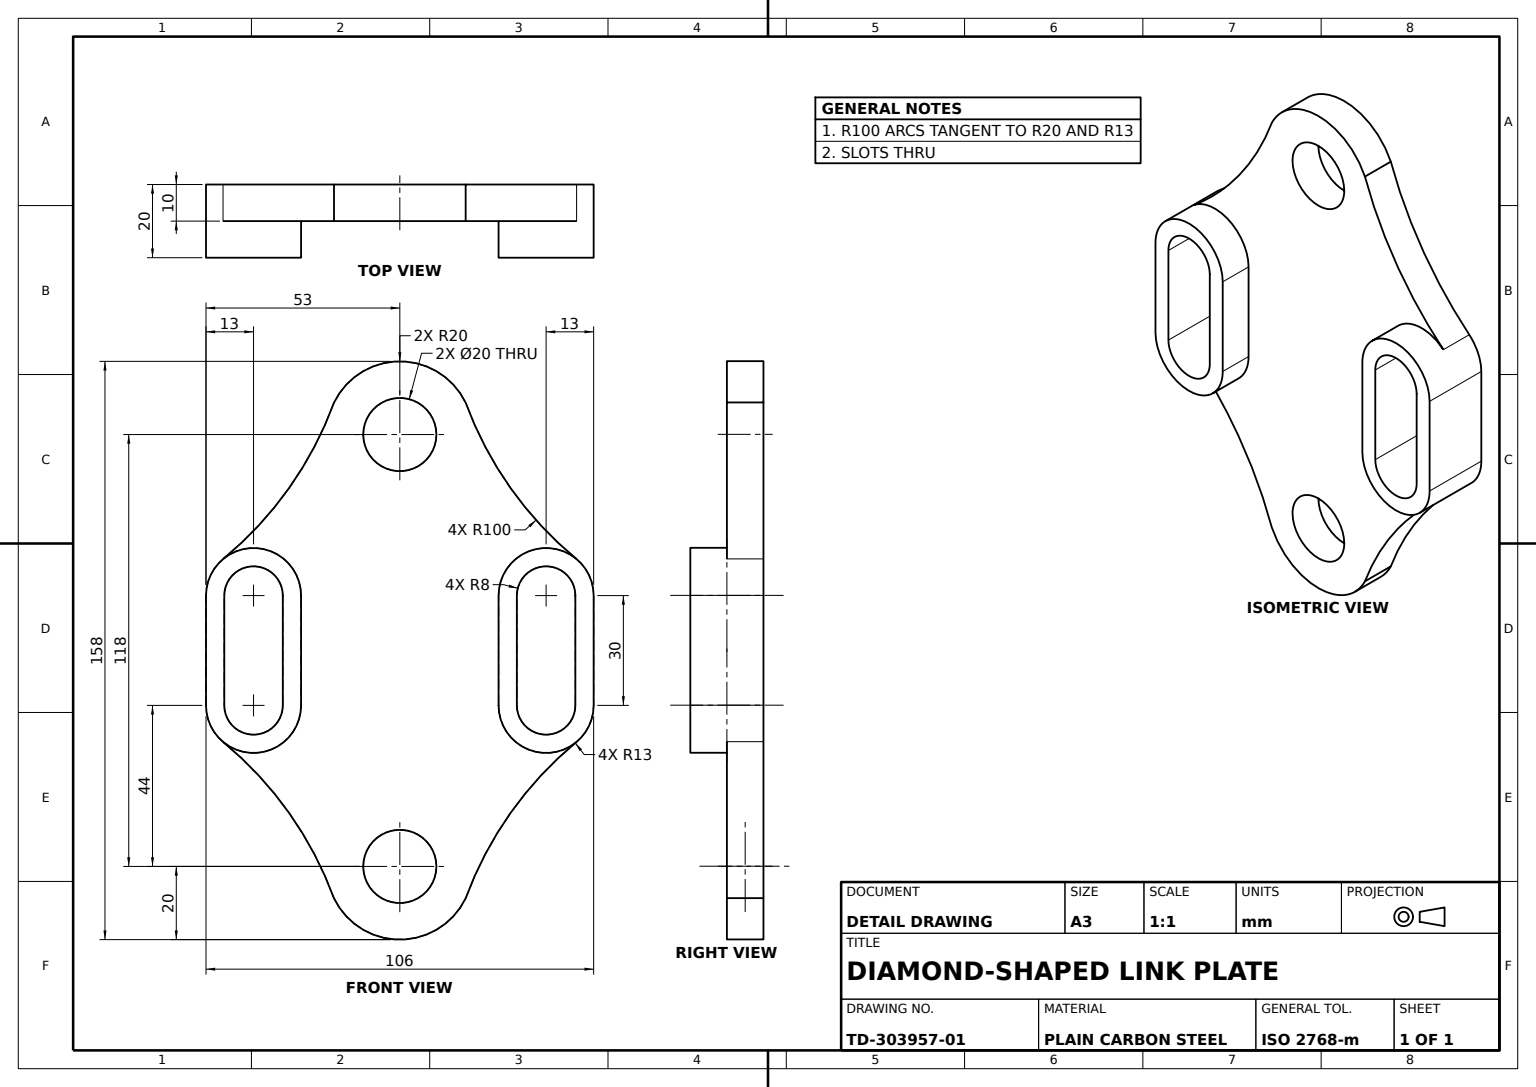
SolidWorks part; units mm, degrees
material "Plain Carbon Steel"
ref_plane "Front Plane" through (0, 0, 0) normal (0, 0, 1) x (1, 0, 0)
ref_plane "Top Plane" through (0, 0, 0) normal (0, 1, 0) x (1, 0, 0)
ref_plane "Right Plane" through (0, 0, 0) normal (1, 0, 0) x (0, 0, -1)
sketch "Diamond Plate Profile" plane through (0, 0, 0) normal (0, 0, 1) x (1, 0, 0)
  line L6 (53, -74) -> (53, -44)
  line L8 (-53, -44) -> (-53, -74)
  arc A0 (17.9996, 8.7185) -> (-17.9996, 8.7185) centre (0, 0) ccw
  arc A1 (-17.9996, -126.7185) -> (17.9996, -126.7185) centre (0, -118) ccw
  arc A2 (53, -44) -> (48.341, -34.0287) centre (40, -44) ccw
  arc A3 (48.341, -83.9713) -> (53, -74) centre (40, -74) ccw
  arc A4 (-48.341, -34.0287) -> (-53, -44) centre (-40, -44) ccw
  arc A5 (-53, -74) -> (-48.1941, -84.0924) centre (-40, -74) ccw
  arc A6 (17.9996, 8.7185) -> (48.341, -34.0287) centre (111.866, 43.202) ccw
  arc A7 (-17.9996, 8.7185) -> (-48.341, -34.0287) centre (-111.866, 43.202) cw
  arc A8 (-17.9996, -126.7185) -> (-48.341, -83.9713) centre (-111.866, -161.202) ccw
  arc A9 (17.9996, -126.7185) -> (48.341, -83.9713) centre (111.866, -161.202) cw
  dimension "D1" = 20
  dimension "D2" = 13
  dimension "D3" = 100
  dimension "D4" = 4.659
  dimension "D5" = 35.0004
  dimension "D6" = 53
  dimension "D7" = 164.866
  dimension "D8" = 117.202
extrude "Diamond Plate" add sketch "Diamond Plate Profile" along normal blind 10 contours A1 A9 A3 L6 A2 A6 A0 A7 A4 L8 A5 A8
sketch "Slot Cuts Profile" plane through (0, 0, 10) normal (0, 0, 1) x (1, 0, 0)
  line L0 (-48, -44) -> (-48, -74)
  line L1 (32, -44) -> (32, -74)
  line L2 (-32, -74) -> (-32, -44)
  line L4 (48, -74) -> (48, -44)
  arc A0 (-32, -44) -> (-48, -44) centre (-40, -44) ccw
  arc A2 (48, -44) -> (32, -44) centre (40, -44) ccw
  arc A3 (32, -74) -> (48, -74) centre (40, -74) ccw
  arc A4 (-48, -74) -> (-32, -74) centre (-40, -74) ccw
  dimension "D1" = 8
extrude "Through Slots 2x" cut sketch "Slot Cuts Profile" against normal blind 10
sketch "Slot Boss A Profile" plane through (0, 0, 10) normal (0, 0, 1) x (1, 0, 0)
  line L0 (-27, -44) -> (-27, -74)
  line L2 (-53, -74) -> (-53, -44)
  line L3 (-32, -44) -> (-32, -74)
  line L4 (-48, -44) -> (-48, -74)
  arc A0 (-27, -44) -> (-53, -44) centre (-40, -44) ccw
  arc A1 (-53, -74) -> (-27, -74) centre (-40, -74) ccw
  arc A2 (-32, -44) -> (-48, -44) centre (-40, -44) ccw
  arc A3 (-48, -74) -> (-32, -74) centre (-40, -74) ccw
extrude "Slot Boss A" add sketch "Slot Boss A Profile" along normal blind 10
sketch "End Holes Profile" plane through (0, 0, 10) normal (0, 0, 1) x (1, 0, 0)
  circle A0 centre (0, 0) radius 10
  circle A1 centre (0, -118) radius 10
  dimension "D1" = 20
extrude "End Holes 2x" cut sketch "End Holes Profile" against normal blind 10
sketch "Slot Boss B Profile" plane through (0, 0, 10) normal (0, 0, 1) x (1, 0, 0)
  line L0 (27, -44) -> (27, -74)
  line L2 (53, -74) -> (53, -44)
  line L3 (32, -44) -> (32, -74)
  line L4 (48, -74) -> (48, -44)
  arc A0 (53, -44) -> (27, -44) centre (40, -44) ccw
  arc A1 (27, -74) -> (53, -74) centre (40, -74) ccw
  arc A2 (48, -44) -> (32, -44) centre (40, -44) ccw
  arc A3 (32, -74) -> (48, -74) centre (40, -74) ccw
extrude "Slot Boss B" add sketch "Slot Boss B Profile" along normal blind 10
